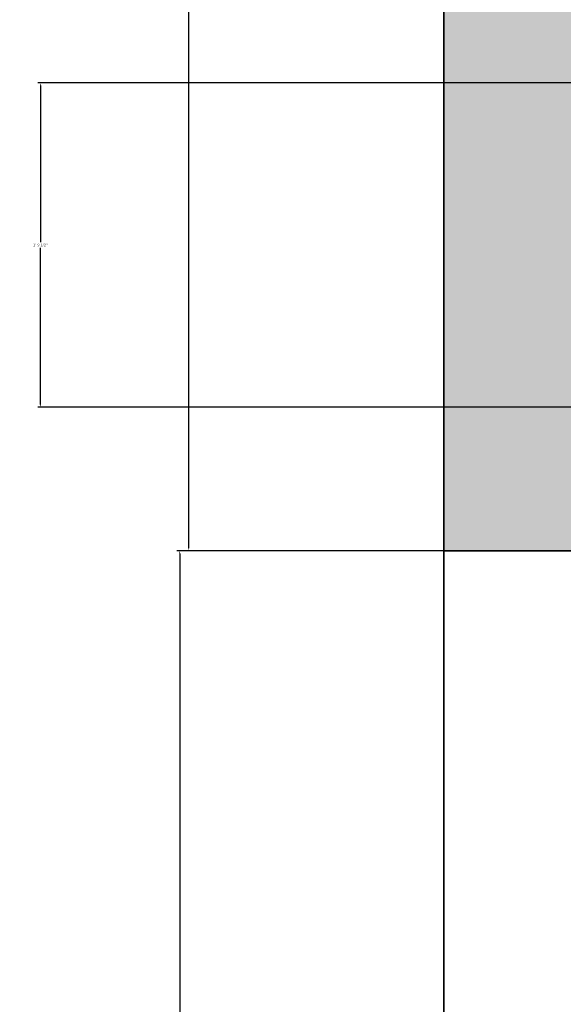
# Model space of a CAD drawing. Units: inches. Extents: x -5 to 330, y -522 to 40.
# Tile 3 of 23: x -5 to 32, y -457 to -391. Entities that reach past the tile are written whole.
import ezdxf

# ---------------------------------------------------------------- set-up
doc = ezdxf.new("R2010")
doc.units = ezdxf.units.IN
doc.header["$MEASUREMENT"] = 0
doc.layers.add('A-ANNO-DIMS', color=2, linetype='Continuous', lineweight=18)
doc.layers.add('A-WALL', color=7, linetype='Continuous', lineweight=35)
doc.layers.add('A-WALL-PATT', color=18, linetype='Continuous', lineweight=13, true_color=0x000000)
doc.styles.get("Standard").update_dxf_attribs({"font": 'arial.ttf'})
doc.dimstyles.get("Standard").update_dxf_attribs({"dimtxt": 0.18, "dimasz": 0.18, "dimexe": 0.18, "dimexo": 0.0625, "dimgap": 0.09, "dimtad": 0, "dimtih": 1, "dimtoh": 1, "dimdec": 0, "dimzin": 0, "dimdsep": 46, "dimlunit": 3, "dimtxsty": 'Standard', "dimcen": 0.09, "dimadec": 0, "dimazin": 0, "dimtfac": 1, "dimtdec": 0, "dimtofl": 0, "dimtmove": 0, "dimatfit": 3, "dimfxl": 1, "dimtolj": 1, "dimtzin": 0, "dimarcsym": 0})

# ---------------------------------------------------------------- blocks, each defined once
blk = doc.blocks.new('*D2')
at = {"layer": 'A-ANNO-DIMS', "color": 0, "lineweight": -2, "transparency": 16777216}
for p, q in [((23.447, 12.356), (6.274, 12.356)), ((6.454, 12.176), (6.454, -203.738)), ((6.454, -425.964), (6.454, -210.049)), ((23.447, -426.144), (6.274, -426.144))]:
    blk.add_line(p, q, dxfattribs=at)
at = {"layer": 'A-ANNO-DIMS', "color": 0, "transparency": 16777216}
for points in [[(6.424, 12.176), (6.484, 12.176), (6.454, 12.356)], [(6.424, -425.964), (6.484, -425.964), (6.454, -426.144)]]:
    blk.add_solid(points, dxfattribs=at)
at = {"layer": 'Defpoints', "color": 0, "transparency": 16777216}
for p in [(23.51, 12.356), (6.454, -426.144), (23.51, -426.144)]:
    blk.add_point(p, dxfattribs=at)
at = {"layer": 'A-ANNO-DIMS', "color": 0, "transparency": 16777216, "insert": (6.454, -206.894), "char_height": 6, "attachment_point": 5}
blk.add_mtext('\\A1;36\'-7"', dxfattribs=at)
blk = doc.blocks.new('*D3')
at = {"layer": 'A-ANNO-DIMS', "color": 0, "lineweight": -2, "transparency": 16777216}
for p, q in [((23.447, -426.144), (5.666, -426.144)), ((5.846, -426.324), (5.846, -457.49)), ((5.846, -494.964), (5.846, -463.797)), ((23.447, -495.144), (5.666, -495.144))]:
    blk.add_line(p, q, dxfattribs=at)
at = {"layer": 'A-ANNO-DIMS', "color": 0, "transparency": 16777216}
for points in [[(5.816, -426.324), (5.876, -426.324), (5.846, -426.144)], [(5.816, -494.964), (5.876, -494.964), (5.846, -495.144)]]:
    blk.add_solid(points, dxfattribs=at)
at = {"layer": 'Defpoints', "color": 0, "transparency": 16777216}
for p in [(23.51, -426.144), (5.846, -495.144), (23.51, -495.144)]:
    blk.add_point(p, dxfattribs=at)
at = {"layer": 'A-ANNO-DIMS', "color": 0, "transparency": 16777216, "insert": (5.846, -460.644), "char_height": 6, "attachment_point": 5}
blk.add_mtext('\\A1;5\'-9"', dxfattribs=at)
blk = doc.blocks.new('*D49')
at = {"layer": 'A-ANNO-DIMS', "color": 0, "lineweight": -2, "transparency": 16777216}
for p, q in [((62.948, -394.834), (-3.655, -394.834)), ((-3.475, -395.014), (-3.475, -405.506)), ((-3.475, -416.364), (-3.475, -405.872)), ((62.948, -416.544), (-3.655, -416.544))]:
    blk.add_line(p, q, dxfattribs=at)
at = {"layer": 'A-ANNO-DIMS', "color": 0, "transparency": 16777216}
for points in [[(-3.505, -395.014), (-3.445, -395.014), (-3.475, -394.834)], [(-3.505, -416.364), (-3.445, -416.364), (-3.475, -416.544)]]:
    blk.add_solid(points, dxfattribs=at)
at = {"layer": 'Defpoints', "color": 0, "transparency": 16777216}
for p in [(63.01, -394.834), (-3.475, -416.544), (63.01, -416.544)]:
    blk.add_point(p, dxfattribs=at)
at = {"layer": 'A-ANNO-DIMS', "color": 0, "transparency": 16777216, "insert": (-3.475, -405.689), "char_height": 0.18, "attachment_point": 5}
blk.add_mtext('\\A1;1\'-9 1/2"', dxfattribs=at)
blk = doc.blocks.new('*D50')
at = {"layer": 'A-ANNO-DIMS', "color": 0, "lineweight": -2, "transparency": 16777216}
for p, q in [((32.51, -417.206), (32.51, -522.309)), ((23.51, -426.206), (23.51, -522.309)), ((23.69, -522.129), (27.681, -522.129)), ((32.33, -522.129), (28.339, -522.129))]:
    blk.add_line(p, q, dxfattribs=at)
at = {"layer": 'A-ANNO-DIMS', "color": 0, "transparency": 16777216}
for points in [[(23.69, -522.099), (23.69, -522.159), (23.51, -522.129)], [(32.33, -522.099), (32.33, -522.159), (32.51, -522.129)]]:
    blk.add_solid(points, dxfattribs=at)
at = {"layer": 'Defpoints', "color": 0, "transparency": 16777216}
for p in [(32.51, -417.144), (23.51, -426.144), (32.51, -522.129)]:
    blk.add_point(p, dxfattribs=at)
at = {"layer": 'A-ANNO-DIMS', "color": 0, "transparency": 16777216, "insert": (28.01, -522.129), "char_height": 0.18, "attachment_point": 5}
blk.add_mtext('\\A1;0\'-9"', dxfattribs=at)

msp = doc.modelspace()

# ---------------------------------------------------------------- hatches: boundary and pattern name
at = {"layer": 'A-WALL-PATT'}
h = msp.add_hatch(color=256, dxfattribs=at)
h.dxf.hatch_style = 1
h.paths.add_polyline_path([(164.01, -44.152), (159.51, -44.152), (159.51, -153.144), (164.01, -153.144)], flags=17)
h.paths.add_polyline_path([(224.01, -188.144), (272.01, -188.144), (272.01, -218.144), (260.01, -218.144), (260.01, -222.644), (272.01, -222.644), (272.01, -292.644), (159.01, -292.644), (159.01, -297.144), (272.01, -297.144), (272.01, -417.144), (245.51, -417.144), (245.51, -426.144), (272.01, -426.144), (272.01, -495.144), (281.01, -495.144), (281.01, 12.356), (23.51, 12.356), (23.51, -426.144), (62.918, -426.144), (62.918, -417.144), (32.51, -417.144), (32.51, -297.144), (48.129, -297.144), (48.129, -292.644), (32.51, -292.644), (32.51, -140.644), (133.51, -140.644), (133.51, -131.644), (32.51, -131.644), (32.51, 3.356), (159.51, 3.356), (164.01, 3.356), (220.01, 3.356), (224.51, 3.356), (272.01, 3.356), (272.01, -179.144), (159.51, -179.144), (159.51, -188.144), (219.51, -188.144), (219.51, -266.644), (224.01, -266.644), (224.01, -222.644), (236.01, -222.644), (236.01, -218.144), (224.01, -218.144)])
h.paths.add_polyline_path([(133.01, -292.644), (128.51, -292.644), (128.51, -297.144), (128.51, -417.144), (122.918, -417.144), (122.918, -426.144), (133.01, -426.144)], flags=17)
h.paths.add_polyline_path([(185.51, -417.144), (159.01, -417.144), (159.01, -426.144), (185.51, -426.144)], flags=17)
h.paths.add_polyline_path([(133.51, -140.644), (129.01, -140.644), (129.01, -246.644), (133.51, -246.644)], flags=17)
h.paths.add_polyline_path([(246.01, -48.644), (224.51, -48.644), (224.51, -27.627), (220.01, -27.627), (220.01, -48.644), (198.604, -48.644), (198.604, -53.144), (246.01, -53.144)], flags=17)

# ---------------------------------------------------------------- linework, layer by layer
at = {"layer": 'A-WALL'}
for p, q in [((23.51, 12.356), (23.51, -495.144)), ((23.51, -426.144), (135.01, -426.144))]:
    msp.add_line(p, q, dxfattribs=at)

# ---------------------------------------------------------------- dimensions: what is measured, and where the dimension line sits
at = {"layer": 'A-ANNO-DIMS'}
for base, p1, p2, override, picture, middle in [((6.454321893, -426.143582029), (23.509888577, 12.356417971), (23.509888577, -426.143582029), {"dimtxt": 6, "dimclrd": 0, "dimclre": 0, "dimclrt": 0}, '*D2', (6.454321893, -206.893582029)), ((-3.475, -416.544), (63.01, -394.834), (63.01, -416.544), {"dimdec": 1, "dimlfac": 1, "dimrnd": 0, "dimzin": 1, "dimdsep": 46, "dimlunit": 4, "dimfrac": 2}, '*D49', (-3.475, -405.689)), ((5.846, -495.144), (23.51, -426.144), (23.51, -495.144), {"dimtxt": 6, "dimclrd": 0, "dimclre": 0, "dimclrt": 0}, '*D3', (5.846, -460.644))]:
    dim = msp.add_linear_dim(base=base, p1=p1, p2=p2, angle=90, dimstyle='Standard', override=override, dxfattribs=at)
    dim.commit()
    dim.dimension.update_dxf_attribs({"geometry": picture, "text_midpoint": middle})
dim = msp.add_linear_dim(base=(32.51, -522.129), p1=(23.51, -426.144), p2=(32.51, -417.144), dimstyle='Standard', override={"dimdec": 1, "dimlfac": 1, "dimrnd": 0, "dimzin": 1, "dimdsep": 46, "dimlunit": 4, "dimfrac": 2}, dxfattribs=at)
dim.commit()
dim.dimension.update_dxf_attribs({"geometry": '*D50', "text_midpoint": (28.01, -522.129)})

doc.saveas('drawing.dxf')
